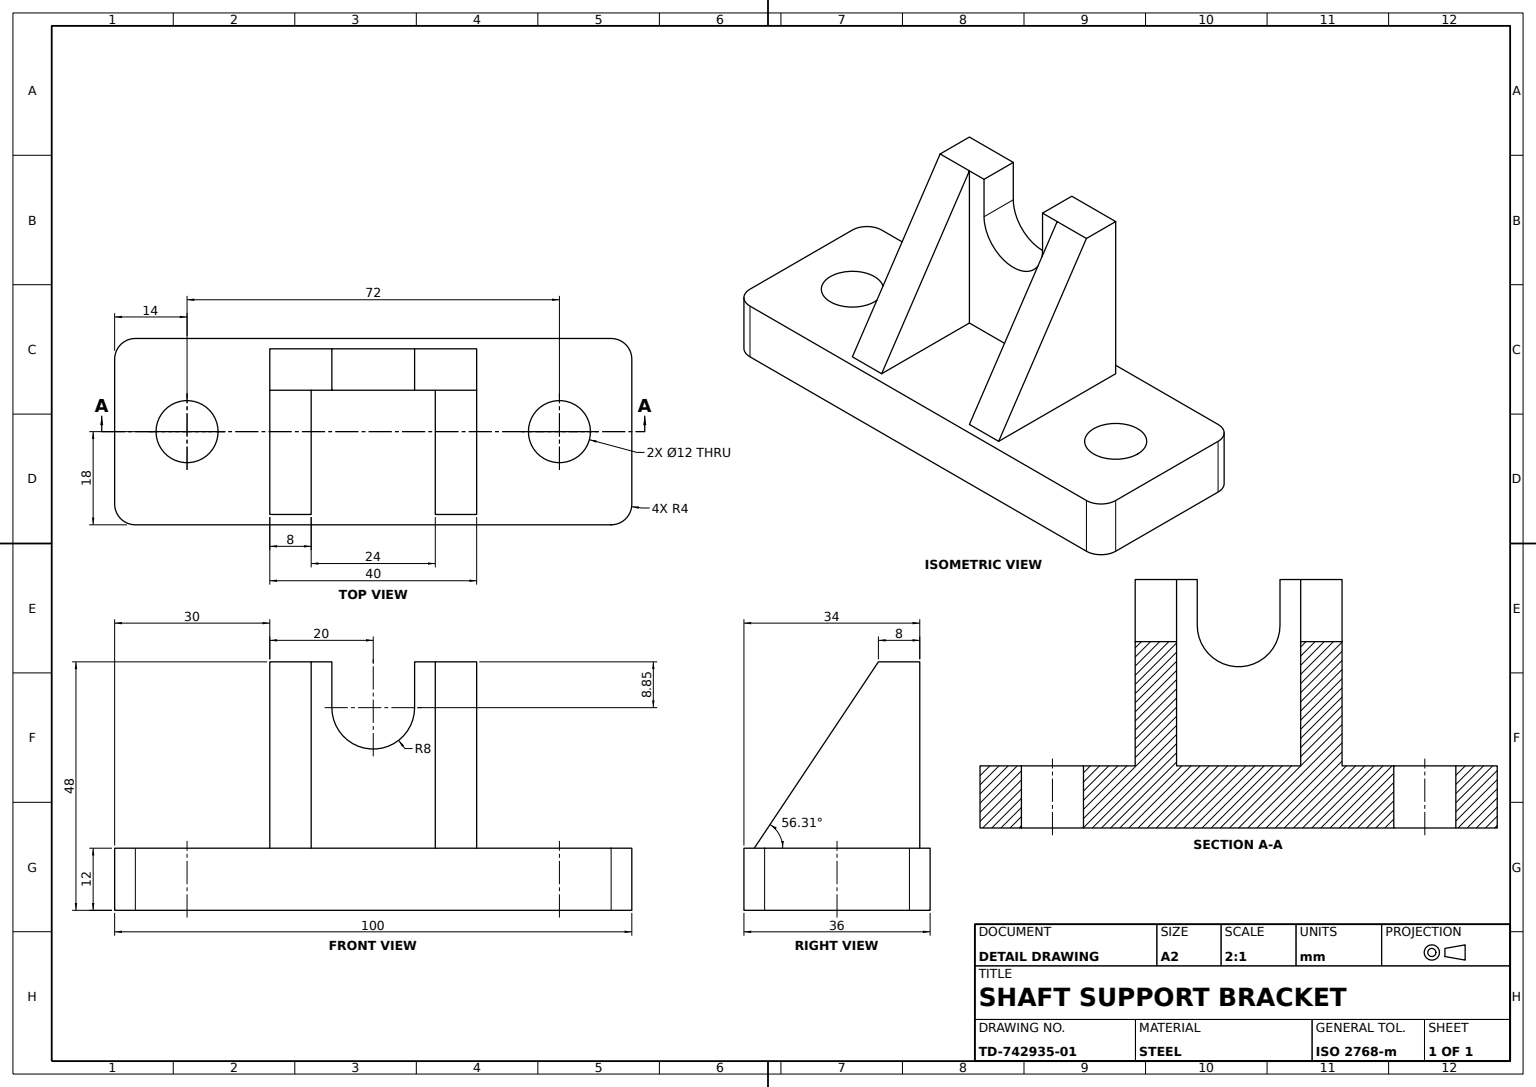
from build123d import *

# Parameters (mm, degrees)
BASE_PLATE_DEPTH                      = 18
BASE_CORNERS_AND_MOUNTING_HOLES_DEPTH = 36
BASE_RELIEF_SKETCH_R                  = 6
BASE_RELIEF_CUT_DEPTH                 = 36
SUPPORT_UPRIGHT_DEPTH                 = 34
UPRIGHT_TAPER_CUT_DEPTH               = 87.764047854
BEARING_SEAT_CUT_DEPTH                = 12


with BuildPart() as part:
    # Base Plate Profile → Base Plate (new, symmetric)
    with BuildSketch(Plane.XY):
        Polygon((0, 0), (50, 0), (50, 12), (-50, 12), (-50, 0), align=None)
    extrude(amount=BASE_PLATE_DEPTH, both=True)

    # Base Corners and Holes Sketch → Base Corners and Mounting Holes (cut)
    with BuildSketch(Plane(origin=(0, 12, 0), x_dir=(1, 0, 0), z_dir=(0, 1, 0))):
        with BuildLine():
            Line((-50, -14), (-50, -18))
            Line((-50, -18), (-46, -18))
            ThreePointArc((-46, -18), (-48.828427125, -16.828427125), (-50, -14))
        make_face()
        with BuildLine():
            Line((50, -14), (50, -18))
            Line((50, -18), (46, -18))
            ThreePointArc((46, -18), (48.828427125, -16.828427125), (50, -14))
        make_face()
        with BuildLine():
            Line((50, 14), (50, 18))
            Line((50, 18), (46, 18))
            ThreePointArc((46, 18), (48.828427125, 16.828427125), (50, 14))
        make_face()
        with BuildLine():
            Line((-50, 18), (-46, 18))
            ThreePointArc((-46, 18), (-48.828427125, 16.828427125), (-50, 14))
            Line((-50, 14), (-50, 18))
        make_face()
    extrude(amount=-BASE_CORNERS_AND_MOUNTING_HOLES_DEPTH, mode=Mode.SUBTRACT)

    # Base Relief Sketch → Base Relief Cut (cut)
    with BuildSketch(Plane(origin=(0, 12, 0), x_dir=(1, 0, 0), z_dir=(0, 1, 0))):
        with Locations(Location((-36, 0, 0), (0, 0, 180))):
            Circle(BASE_RELIEF_SKETCH_R)
        with Locations(Location((36, 0, 0), (0, 0, 270))):
            Circle(BASE_RELIEF_SKETCH_R)
    extrude(amount=-BASE_RELIEF_CUT_DEPTH, mode=Mode.SUBTRACT)

    # Upright Profile → Support Upright (add)
    with BuildSketch(Plane.XY.offset(18)):
        with BuildLine():
            Line((8, 39.150951317), (8, 48))
            Line((8, 48), (20, 48))
            Line((20, 48), (20, 12))
            Line((20, 12), (-20, 12))
            Line((-20, 12), (-20, 48))
            Line((-20, 48), (-8, 48))
            Line((-8, 48), (-8, 39.150951317))
            ThreePointArc((-8, 39.150951317), (0, 31.150951317), (8, 39.150951317))
        make_face()
    extrude(amount=-SUPPORT_UPRIGHT_DEPTH)

    # Upright Taper Sketch → Upright Taper Cut (cut, through all)
    with BuildSketch(Plane.ZY.offset(20)):
        Polygon((-8, 48), (18, 48), (18, 12), (16, 12), align=None)
    extrude(amount=-UPRIGHT_TAPER_CUT_DEPTH, mode=Mode.SUBTRACT)

    # Bearing Seat Sketch → Bearing Seat Cut (cut, symmetric)
    with BuildSketch(Plane(origin=(0, 0, 0), x_dir=(0, 0, -1), z_dir=(1, 0, 0))):
        Polygon((8, 48), (8, 12), (-16, 12), align=None)
    extrude(amount=BEARING_SEAT_CUT_DEPTH, both=True, mode=Mode.SUBTRACT)


solid = part.part
